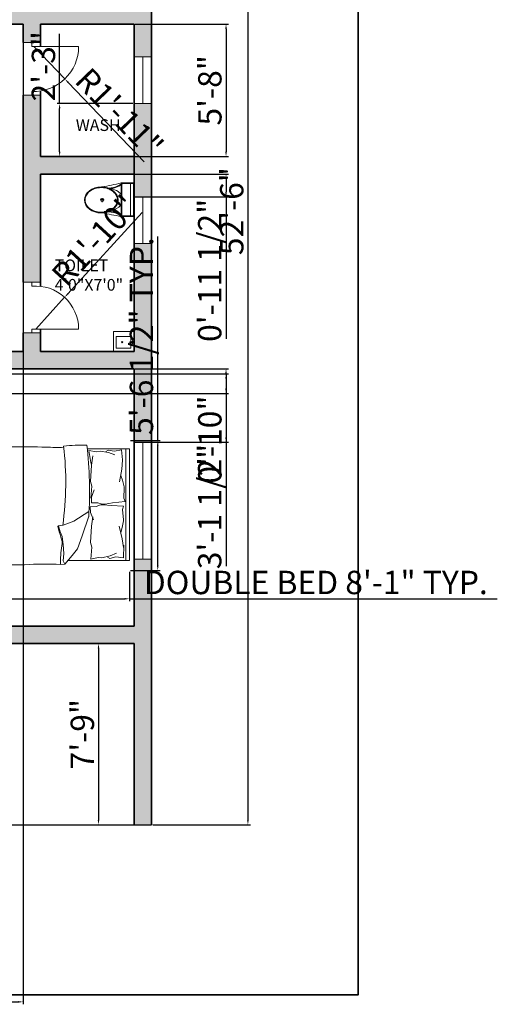
# Model space of a CAD drawing. Units: inches. Extents: x 995 to 1625, y 1005 to 1825.
# Tile 4 of 5: x 1379 to 1625, y 1015 to 1521. Entities that reach past the tile are written whole.
import ezdxf

# ---------------------------------------------------------------- set-up
doc = ezdxf.new("R2010")
doc.units = ezdxf.units.IN
for name, color, linetype, lineweight in [('A-ANNO-DIMS', 2, 'Continuous', 18), ('A-ANNO-TTLB', 7, 'Continuous', 35), ('A-AREA-IDEN', 7, 'Continuous', 18), ('A-DOOR', 4, 'Continuous', 18), ('A-FLOR-FIXT', 9, 'Continuous', 18), ('A-FURN', 8, 'Continuous', 13), ('A-GLAZ', 3, 'Continuous', 18), ('A-WALL', 7, 'Continuous', 35), ('C-PROP', 7, 'Continuous', 25)]:
    doc.layers.add(name, color=color, linetype=linetype, lineweight=lineweight)
doc.layers.add('A-WALL-PATT', color=251, linetype='Continuous', lineweight=13, true_color=0x636466)
doc.styles.get("Standard").update_dxf_attribs({"font": 'arial.ttf'})
doc.dimstyles.new('ISO-25', dxfattribs={"dimtxt": 12, "dimasz": 2.5, "dimexe": 1.25, "dimexo": 0.625, "dimtad": 1, "dimdec": 0, "dimlunit": 3, "dimtxsty": 'Standard', "dimcen": 2.5, "dimadec": 0, "dimazin": 0, "dimtfac": 1, "dimtdec": 0, "dimtmove": 0, "dimatfit": 3, "dimfxl": 1, "dimarcsym": 0})

# ---------------------------------------------------------------- blocks, each defined once
blk = doc.blocks.new('*D3')
at = {"layer": 'A-ANNO-DIMS', "color": 0, "lineweight": -2, "transparency": 16777216}
for p, q in [((1419.59, 1197.93), (1419.59, 1109.93)), ((1420.21, 1200.43), (1420.84, 1200.43)), ((1420.21, 1107.43), (1420.84, 1107.43))]:
    blk.add_line(p, q, dxfattribs=at)
at = {"layer": 'A-ANNO-DIMS', "color": 0, "transparency": 16777216}
for points in [[(1419.17, 1197.93), (1420, 1197.93), (1419.59, 1200.43)], [(1419.17, 1109.93), (1420, 1109.93), (1419.59, 1107.43)]]:
    blk.add_solid(points, dxfattribs=at)
at = {"layer": 'Defpoints', "color": 0, "transparency": 16777216}
for p in [(1419.59, 1200.43), (1419.59, 1107.43), (1419.59, 1107.43)]:
    blk.add_point(p, dxfattribs=at)
at = {"layer": 'A-ANNO-DIMS', "color": 0, "transparency": 16777216, "insert": (1412.84, 1153.93), "char_height": 12, "attachment_point": 5, "rotation": 90}
blk.add_mtext('7\'-9"', dxfattribs=at)
blk = doc.blocks.new('*D4')
at = {"layer": 'A-ANNO-DIMS', "color": 0, "lineweight": -2, "transparency": 16777216}
for p, q in [((1447.49, 1737.43), (1497.61, 1737.43)), ((1496.36, 1734.93), (1496.36, 1109.93)), ((1447.49, 1107.43), (1497.61, 1107.43))]:
    blk.add_line(p, q, dxfattribs=at)
at = {"layer": 'A-ANNO-DIMS', "color": 0, "transparency": 16777216}
for points in [[(1495.94, 1734.93), (1496.78, 1734.93), (1496.36, 1737.43)], [(1495.94, 1109.93), (1496.78, 1109.93), (1496.36, 1107.43)]]:
    blk.add_solid(points, dxfattribs=at)
at = {"layer": 'Defpoints', "color": 0, "transparency": 16777216}
for p in [(1446.87, 1737.43), (1446.87, 1107.43), (1496.36, 1107.43)]:
    blk.add_point(p, dxfattribs=at)
at = {"layer": 'A-ANNO-DIMS', "color": 0, "transparency": 16777216, "insert": (1489.61, 1422.43), "char_height": 12, "attachment_point": 5, "rotation": 90}
blk.add_mtext('52\'-6"', dxfattribs=at)
blk = doc.blocks.new('A$C31115884')
for p, q in [((283, 498), (223, 498)), ((258, 466), (258, 523)), ((0, 200), (0, 0)), ((520, 200), (0, 200)), ((10, 190), (10, 10)), ((510, 190), (10, 190)), ((510, 10), (510, 190)), ((520, 0), (520, 200)), ((510, 54), (0, 54)), ((10, 10), (510, 10)), ((0, 0), (520, 0))]:
    blk.add_line(p, q)
blk.add_circle((256, 496), 23.6)
for centre, radius, start, end in [((2778, -205), 2807, 165.4549, 171.7133), ((-295, 403), 365, 324.2091, 9.3499), ((-295, 403), 375, 324.2091, 9.3499), ((806, 403), 365, 170.6501, 215.7909), ((3237, 905), 2807, 188.2867, 194.5451), ((384, 406), 293, 190.2774, 224.1564), ((139, 406), 293, 315.8436, 2.6563), ((806, 403), 375, 179.2036, 215.7909)]:
    blk.add_arc(centre, radius, start, end)
blk.add_ellipse((256, 510), major_axis=(0, -261), ratio=0.772727)
blk.add_open_spline([(256, 259), (263, 259), (270, 260), (288, 262), (299, 265), (320, 273), (330, 278), (350, 291), (360, 299), (378, 316), (386, 326), (402, 347), (409, 358), (421, 383), (427, 395), (436, 422), (440, 436), (445, 465), (447, 480), (448, 509), (448, 524), (445, 553), (443, 568), (436, 596), (432, 610), (422, 636), (416, 649), (402, 672), (395, 683), (379, 703), (370, 712), (351, 728), (341, 735), (321, 746), (310, 751), (289, 757), (278, 759), (256, 761), (245, 761), (223, 757), (212, 754), (191, 746), (181, 741), (161, 728), (151, 720), (133, 703), (125, 693), (110, 672), (103, 660), (90, 636), (85, 623), (76, 596), (72, 582), (67, 553), (66, 538), (64, 509), (65, 494), (68, 465), (70, 450), (77, 422), (81, 408), (91, 382), (97, 370), (111, 346), (118, 335), (135, 316), (144, 307), (162, 291), (172, 284), (193, 273), (203, 269), (225, 262), (236, 260), (250, 259), (253, 259), (256, 259)], degree=3, knots=[0, 0, 0, 0, 0.110105, 0.110105, 0.285049, 0.285049, 0.459994, 0.459994, 0.634938, 0.634938, 0.809882, 0.809882, 0.984827, 0.984827, 1.159771, 1.159771, 1.334715, 1.334715, 1.50966, 1.50966, 1.684604, 1.684604, 1.859549, 1.859549, 2.034493, 2.034493, 2.209437, 2.209437, 2.384382, 2.384382, 2.559326, 2.559326, 2.73427, 2.73427, 2.909215, 2.909215, 3.084159, 3.084159, 3.259103, 3.259103, 3.434048, 3.434048, 3.608992, 3.608992, 3.783936, 3.783936, 3.958881, 3.958881, 4.133825, 4.133825, 4.30877, 4.30877, 4.483714, 4.483714, 4.658658, 4.658658, 4.833603, 4.833603, 5.008547, 5.008547, 5.183491, 5.183491, 5.358436, 5.358436, 5.53338, 5.53338, 5.708324, 5.708324, 5.883269, 5.883269, 6.058213, 6.058213, 6.233158, 6.233158, 6.283185, 6.283185, 6.283185, 6.283185])
blk = doc.blocks.new('WIN-24IN')
for p, q in [((0, 0), (0, -9)), ((24, -4.5), (24, 0)), ((24, 0), (24, -9)), ((0, -9), (0, -4.5)), ((0, -4.5), (24, -4.5))]:
    blk.add_line(p, q)
blk = doc.blocks.new('WIN-60IN')
for p, q in [((0, 0), (9, 0)), ((9, 0), (4.5, 0)), ((4.5, 0), (4.5, -60)), ((4.5, -60), (0, -60)), ((0, -60), (9, -60))]:
    blk.add_line(p, q)
blk = doc.blocks.new('BED-DOUBLE')
for p, q in [((13.64, 59.31), (35.36, 59.31)), ((15.43, 52.35), (14.57, 58.46)), ((14.57, 58.46), (18.38, 57.77)), ((16.62, 55.83), (15.82, 50.99)), ((18.38, 57.77), (20.29, 58.11)), ((20.29, 58.11), (24.62, 57.42)), ((24.45, 58.63), (23.23, 57.94)), ((27.57, 58.11), (24.45, 58.63)), ((24.62, 57.42), (27.91, 56.21)), ((31.38, 58.81), (27.57, 58.11)), ((31.35, 58.8), (31.75, 53.67)), ((33.52, 59.31), (33.52, 2.02)), ((35.36, 59.31), (35.36, 2.02)), ((15.82, 50.99), (15.3, 42.59)), ((15.82, 50.99), (15.43, 52.35)), ((31.73, 53.54), (31.38, 48.96)), ((31.75, 53.67), (31.73, 53.54)), ((31.38, 48.96), (30.17, 42.37)), ((30.86, 45.67), (31.73, 43.24)), ((-59.65, 45.42), (-59.65, 15.91)), ((15.3, 42.59), (15.97, 40.24)), ((31.73, 43.24), (32.59, 39.77)), ((15.97, 40.24), (15.49, 34.09)), ((15.86, 34.58), (17.17, 38.35)), ((32.59, 39.39), (32.42, 34.06)), ((32.59, 39.77), (32.59, 39.39)), ((15.86, 31.63), (15.86, 34.58)), ((19.07, 31.63), (15.86, 31.63)), ((20.52, 30.58), (18.31, 29.75)), ((21.33, 30.94), (19.07, 31.63)), ((22.07, 30.68), (20.52, 30.58)), ((22.89, 30.94), (21.33, 30.94)), ((25.92, 30.23), (22.07, 30.68)), ((26.7, 31.63), (22.89, 30.94)), ((33.11, 32.33), (26.7, 31.63)), ((32.42, 34.06), (33.11, 32.33)), ((14.51, 27.2), (6.73, 22.18)), ((18.31, 29.75), (15.1, 29.55)), ((15.1, 29.55), (15.29, 26.61)), ((15.29, 26.61), (16.83, 22.93)), ((32.37, 29.94), (25.92, 30.23)), ((31.78, 28.16), (32.37, 29.94)), ((32.29, 22.85), (31.78, 28.16)), ((6.73, 22.18), (1.35, 20.13)), ((11, 14.75), (14.51, 24.75)), ((16.62, 24.44), (15.82, 19.6)), ((31.66, 18.96), (32.31, 22.47)), ((32.31, 22.47), (32.29, 22.85)), ((1.35, 20.13), (-1.06, 19.76)), ((-1.06, 19.76), (-0.32, 16.79)), ((-0.32, 16.79), (0.79, 14.38)), ((15.82, 19.6), (15.3, 11.2)), ((31.68, 13.23), (30.05, 19.72)), ((30.95, 16.48), (31.66, 18.96)), ((0.79, 14.38), (1.35, 10.29)), ((1.35, 10.29), (1.72, 5.65)), ((8.59, 8.07), (11, 14.75)), ((15.3, 11.2), (15.97, 8.85)), ((32.31, 8.67), (31.68, 13.23)), ((1.72, 5.65), (1.35, 1.94)), ((5.99, 4.54), (8.59, 8.07)), ((15.97, 8.85), (15.49, 2.7)), ((25.46, 4.36), (28.67, 5.78)), ((32.29, 3.4), (32.41, 9.88)), ((32.41, 9.88), (32.31, 8.67)), ((0, 0), (2.09, 0.1, 4.64)), ((1.35, 1.94), (2.09, 0.1)), ((2.09, 0.1), (5.99, 4.54)), ((35.36, 2.02), (3.45, 2.02)), ((15.49, 2.7), (19.25, 3.63)), ((19.25, 3.63), (21.17, 3.4)), ((21.17, 3.4), (25.46, 4.36)), ((25.36, 3.14), (24.1, 3.76)), ((28.44, 3.85), (25.36, 3.14)), ((32.29, 3.4), (28.44, 3.85))]:
    blk.add_line(p, q)
for centre, radius, start, end in [((-60.22, 62.17), 1.31, 56.1736, 203.4781), ((-205.42, 37.79), 145.97, 2.9958, 9.4091), ((-48.9, 89.44), 28.25, 247.9751, 266.652), ((-41.99, 95.72), 35.53, 256.0648, 268.9113), ((-152.05, 42.19), 154.68, 351.7845, 6.9006), ((11.26, -38.62), 99.87, 88.7218, 95.604), ((-182.9, 37.87), 197.77, 356.0865, 6.7821), ((-25.32, -517.76), 578.22, 88.22771, 91.71854), ((-2.02, 264.05), 203.94, 268.4762, 271.0082), ((63.78, 84.12), 127.63, 193.3832, 197.7053), ((-219.13, 14.14), 159.5, 354.4998, 0.6351), ((-1.14, 19.55), 0.221, 70.2464, 181.1377), ((33.58, 26.13), 35.55, 190.6617, 199.8806), ((-6.68, 11.03), 7.46, 348.6608, 23.7384), ((43.33, 1.94), 43.38, 169.8763, 182.5657), ((-8.18, -155.03), 155.25, 86.9791, 93.8365), ((-46.97, -27.83), 27.65, 87.4714, 116.4681), ((-45.95, 5468.82), 5469.02, 270.00217, 270.28689)]:
    blk.add_arc(centre, radius, start, end)
blk = doc.blocks.new('*D18')
at = {"layer": 'A-ANNO-DIMS', "color": 0, "lineweight": -2, "transparency": 16777216}
for p, q in [((1338.5, 1237.34), (1338.5, 1222.16)), ((1435.5, 1237.34), (1435.5, 1222.16)), ((1341, 1223.41), (1433, 1223.41)), ((1435.5, 1223.41), (1624.52, 1223.41))]:
    blk.add_line(p, q, dxfattribs=at)
at = {"layer": 'A-ANNO-DIMS', "color": 0, "transparency": 16777216}
for points in [[(1341, 1223.83), (1341, 1223), (1338.5, 1223.41)], [(1433, 1223.83), (1433, 1223), (1435.5, 1223.41)]]:
    blk.add_solid(points, dxfattribs=at)
at = {"layer": 'Defpoints', "color": 0, "transparency": 16777216}
for p in [(1338.5, 1237.96), (1435.5, 1237.96), (1435.5, 1223.41)]:
    blk.add_point(p, dxfattribs=at)
at = {"layer": 'A-ANNO-DIMS', "color": 0, "transparency": 16777216, "insert": (1531.26, 1230.25), "char_height": 12, "attachment_point": 5}
blk.add_mtext('DOUBLE BED 8\'-1" TYP.', dxfattribs=at)
blk = doc.blocks.new('*D19')
at = {"layer": 'A-ANNO-DIMS', "color": 0, "lineweight": -2, "transparency": 16777216}
for p, q in [((1450.05, 1304.62), (1450.05, 1409.47)), ((1436.12, 1304.62), (1451.3, 1304.62)), ((1450.05, 1240.46), (1450.05, 1302.12)), ((1436.12, 1237.96), (1451.3, 1237.96))]:
    blk.add_line(p, q, dxfattribs=at)
at = {"layer": 'A-ANNO-DIMS', "color": 0, "transparency": 16777216}
for points in [[(1449.63, 1302.12), (1450.46, 1302.12), (1450.05, 1304.62)], [(1449.63, 1240.46), (1450.46, 1240.46), (1450.05, 1237.96)]]:
    blk.add_solid(points, dxfattribs=at)
at = {"layer": 'Defpoints', "color": 0, "transparency": 16777216}
for p in [(1435.5, 1304.62), (1450.05, 1304.62), (1435.5, 1237.96)]:
    blk.add_point(p, dxfattribs=at)
at = {"layer": 'A-ANNO-DIMS', "color": 0, "transparency": 16777216, "insert": (1443.22, 1358.29), "char_height": 12, "attachment_point": 5, "rotation": 90}
blk.add_mtext('5\'-6 1/2" TYP.', dxfattribs=at)
blk = doc.blocks.new('*D26')
at = {"layer": 'A-ANNO-DIMS', "color": 0, "lineweight": -2, "transparency": 16777216}
for p, q in [((1076.49, 1338.88), (1486.37, 1338.88)), ((1485.12, 1336.38), (1485.12, 1331.38)), ((1076.49, 1328.88), (1486.37, 1328.88)), ((1485.12, 1328.88), (1485.12, 1283.91))]:
    blk.add_line(p, q, dxfattribs=at)
at = {"layer": 'A-ANNO-DIMS', "color": 0, "transparency": 16777216}
for points in [[(1484.7, 1336.38), (1485.53, 1336.38), (1485.12, 1338.88)], [(1484.7, 1331.38), (1485.53, 1331.38), (1485.12, 1328.88)]]:
    blk.add_solid(points, dxfattribs=at)
at = {"layer": 'Defpoints', "color": 0, "transparency": 16777216}
for p in [(1075.87, 1338.88), (1075.87, 1328.88), (1485.12, 1328.88)]:
    blk.add_point(p, dxfattribs=at)
at = {"layer": 'A-ANNO-DIMS', "color": 0, "transparency": 16777216, "insert": (1478.36, 1305.15), "char_height": 12, "attachment_point": 5, "rotation": 90}
blk.add_mtext('0\'-10"', dxfattribs=at)
blk = doc.blocks.new('*D28')
at = {"layer": 'A-ANNO-DIMS', "color": 0, "lineweight": -2, "transparency": 16777216}
for p, q in [((1438.49, 1518.43), (1486.37, 1518.43)), ((1485.12, 1515.93), (1485.12, 1452.93)), ((1438.49, 1450.43), (1486.37, 1450.43))]:
    blk.add_line(p, q, dxfattribs=at)
at = {"layer": 'A-ANNO-DIMS', "color": 0, "transparency": 16777216}
for points in [[(1484.7, 1515.93), (1485.53, 1515.93), (1485.12, 1518.43)], [(1484.7, 1452.93), (1485.53, 1452.93), (1485.12, 1450.43)]]:
    blk.add_solid(points, dxfattribs=at)
at = {"layer": 'Defpoints', "color": 0, "transparency": 16777216}
for p in [(1437.87, 1518.43), (1437.87, 1450.43), (1485.12, 1450.43)]:
    blk.add_point(p, dxfattribs=at)
at = {"layer": 'A-ANNO-DIMS', "color": 0, "transparency": 16777216, "insert": (1478.36, 1484.43), "char_height": 12, "attachment_point": 5, "rotation": 90}
blk.add_mtext('5\'-8"', dxfattribs=at)
blk = doc.blocks.new('*D29')
at = {"layer": 'A-ANNO-DIMS', "color": 0, "lineweight": -2, "transparency": 16777216}
for p, q in [((1380.24, 1518.43), (1341.37, 1518.43)), ((1342.62, 1352.93), (1342.62, 1515.93)), ((1380.24, 1350.43), (1341.37, 1350.43))]:
    blk.add_line(p, q, dxfattribs=at)
at = {"layer": 'A-ANNO-DIMS', "color": 0, "transparency": 16777216}
for points in [[(1342.2, 1515.93), (1343.03, 1515.93), (1342.62, 1518.43)], [(1342.2, 1352.93), (1343.03, 1352.93), (1342.62, 1350.43)]]:
    blk.add_solid(points, dxfattribs=at)
at = {"layer": 'Defpoints', "color": 0, "transparency": 16777216}
for p in [(1342.62, 1518.43), (1380.87, 1518.43), (1380.87, 1350.43)]:
    blk.add_point(p, dxfattribs=at)
at = {"layer": 'A-ANNO-DIMS', "color": 0, "transparency": 16777216, "insert": (1335.86, 1434.43), "char_height": 12, "attachment_point": 5, "rotation": 90}
blk.add_mtext('14\'-0"', dxfattribs=at)
blk = doc.blocks.new('*D30')
at = {"layer": 'A-ANNO-DIMS', "color": 0, "lineweight": -2, "transparency": 16777216}
for p, q in [((1212.87, 1517.8), (1212.87, 1015.27)), ((1380.87, 1517.8), (1380.87, 1015.27)), ((1215.37, 1016.52), (1378.37, 1016.52))]:
    blk.add_line(p, q, dxfattribs=at)
at = {"layer": 'A-ANNO-DIMS', "color": 0, "transparency": 16777216}
for points in [[(1215.37, 1016.93), (1215.37, 1016.1), (1212.87, 1016.52)], [(1378.37, 1016.93), (1378.37, 1016.1), (1380.87, 1016.52)]]:
    blk.add_solid(points, dxfattribs=at)
at = {"layer": 'Defpoints', "color": 0, "transparency": 16777216}
for p in [(1212.87, 1518.43), (1380.87, 1518.43), (1380.87, 1016.52)]:
    blk.add_point(p, dxfattribs=at)
at = {"layer": 'A-ANNO-DIMS', "color": 0, "transparency": 16777216, "insert": (1296.87, 1023.27), "char_height": 12, "attachment_point": 5}
blk.add_mtext('14\'-0"', dxfattribs=at)
blk = doc.blocks.new('*D39')
at = {"layer": 'A-ANNO-DIMS', "color": 0, "lineweight": -2, "transparency": 16777216}
for p, q in [((1399.62, 1477.62), (1399.62, 1513.47)), ((1437.24, 1477.62), (1398.37, 1477.62)), ((1399.62, 1452.93), (1399.62, 1475.12)), ((1437.24, 1450.43), (1398.37, 1450.43))]:
    blk.add_line(p, q, dxfattribs=at)
at = {"layer": 'A-ANNO-DIMS', "color": 0, "transparency": 16777216}
for points in [[(1399.2, 1475.12), (1400.03, 1475.12), (1399.62, 1477.62)], [(1399.2, 1452.93), (1400.03, 1452.93), (1399.62, 1450.43)]]:
    blk.add_solid(points, dxfattribs=at)
at = {"layer": 'Defpoints', "color": 0, "transparency": 16777216}
for p in [(1399.62, 1477.62), (1437.87, 1477.62), (1437.87, 1450.43)]:
    blk.add_point(p, dxfattribs=at)
at = {"layer": 'A-ANNO-DIMS', "color": 0, "transparency": 16777216, "insert": (1392.86, 1496.79), "char_height": 12, "attachment_point": 5, "rotation": 90}
blk.add_mtext('2\'-3"', dxfattribs=at)
blk = doc.blocks.new('*D40')
at = {"layer": 'A-ANNO-DIMS', "color": 0, "lineweight": -2, "transparency": 16777216}
for p, q in [((1438.49, 1441.43), (1486.37, 1441.43)), ((1485.12, 1438.93), (1485.12, 1432.25)), ((1438.49, 1429.75), (1486.37, 1429.75)), ((1485.12, 1429.75), (1485.12, 1356.81))]:
    blk.add_line(p, q, dxfattribs=at)
at = {"layer": 'A-ANNO-DIMS', "color": 0, "transparency": 16777216}
for points in [[(1484.7, 1438.93), (1485.53, 1438.93), (1485.12, 1441.43)], [(1484.7, 1432.25), (1485.53, 1432.25), (1485.12, 1429.75)]]:
    blk.add_solid(points, dxfattribs=at)
at = {"layer": 'Defpoints', "color": 0, "transparency": 16777216}
for p in [(1437.87, 1441.43), (1437.87, 1429.75), (1485.12, 1429.75)]:
    blk.add_point(p, dxfattribs=at)
at = {"layer": 'A-ANNO-DIMS', "color": 0, "transparency": 16777216, "insert": (1478.29, 1392.03), "char_height": 12, "attachment_point": 5, "rotation": 90}
blk.add_mtext('0\'-11 1/2"', dxfattribs=at)
blk = doc.blocks.new('*D41')
at = {"layer": 'A-ANNO-DIMS', "color": 0, "lineweight": -2, "transparency": 16777216}
for p, q in [((1438.49, 1341.43), (1486.37, 1341.43)), ((1485.12, 1338.93), (1485.12, 1306.34)), ((1438.49, 1303.84), (1486.37, 1303.84)), ((1485.12, 1303.84), (1485.12, 1240.24))]:
    blk.add_line(p, q, dxfattribs=at)
at = {"layer": 'A-ANNO-DIMS', "color": 0, "transparency": 16777216}
for points in [[(1484.7, 1338.93), (1485.53, 1338.93), (1485.12, 1341.43)], [(1484.7, 1306.34), (1485.53, 1306.34), (1485.12, 1303.84)]]:
    blk.add_solid(points, dxfattribs=at)
at = {"layer": 'Defpoints', "color": 0, "transparency": 16777216}
for p in [(1437.87, 1341.43), (1437.87, 1303.84), (1485.12, 1303.84)]:
    blk.add_point(p, dxfattribs=at)
at = {"layer": 'A-ANNO-DIMS', "color": 0, "transparency": 16777216, "insert": (1478.28, 1270.79), "char_height": 12, "attachment_point": 5, "rotation": 90}
blk.add_mtext('3\'-1 1/2"', dxfattribs=at)
blk = doc.blocks.new('*D51')
at = {"layer": 'A-ANNO-DIMS', "color": 0, "lineweight": -2, "transparency": 16777216}
for p, q in [((1386.31, 1506.92), (1402.28, 1490.28)), ((1443.11, 1447.75), (1404.01, 1488.48))]:
    blk.add_line(p, q, dxfattribs=at)
at = {"layer": 'A-ANNO-DIMS', "color": 0, "transparency": 16777216}
blk.add_solid([(1404.31, 1488.77), (1403.71, 1488.19), (1402.28, 1490.28)], dxfattribs=at)
at = {"layer": 'Defpoints', "color": 0, "transparency": 16777216}
for p in [(1386.31, 1506.92), (1402.28, 1490.28)]:
    blk.add_point(p, dxfattribs=at)
at = {"layer": 'A-ANNO-DIMS', "color": 0, "transparency": 16777216, "insert": (1429.22, 1471.82), "char_height": 12, "attachment_point": 5, "rotation": 313.833}
blk.add_mtext('R1\'-11"', dxfattribs=at)
blk = doc.blocks.new('*D53')
at = {"layer": 'A-ANNO-DIMS', "color": 0, "lineweight": -2, "transparency": 16777216}
for p, q in [((1442.01, 1421.66), (1403.89, 1380.02)), ((1387.31, 1361.9), (1402.2, 1378.17))]:
    blk.add_line(p, q, dxfattribs=at)
at = {"layer": 'A-ANNO-DIMS', "color": 0, "transparency": 16777216}
blk.add_solid([(1403.58, 1380.3), (1404.2, 1379.74), (1402.2, 1378.17)], dxfattribs=at)
at = {"layer": 'Defpoints', "color": 0, "transparency": 16777216}
for p in [(1402.2, 1378.17), (1387.31, 1361.9)]:
    blk.add_point(p, dxfattribs=at)
at = {"layer": 'A-ANNO-DIMS', "color": 0, "transparency": 16777216, "insert": (1418.82, 1406.32), "char_height": 12, "attachment_point": 5, "rotation": 47.5256}
blk.add_mtext('R1\'-10"', dxfattribs=at)

msp = doc.modelspace()

# ---------------------------------------------------------------- hatches: boundary and pattern name
at = {"layer": 'A-WALL-PATT'}
h = msp.add_hatch(color=256, dxfattribs=at)
h.dxf.hatch_style = 1
h.paths.add_polyline_path([(1446.87, 1737.43), (1066.87, 1737.43), (1066.87, 1718.28), (1075.87, 1718.28), (1075.87, 1728.43), (1171.87, 1728.43), (1171.87, 1668.43), (1165.05, 1668.43), (1165.05, 1659.43), (1219.13, 1659.43), (1219.13, 1663.93), (1219.13, 1668.43), (1180.87, 1668.43), (1180.87, 1691.88), (1180.87, 1728.43), (1249.87, 1728.43), (1258.87, 1728.43), (1332.87, 1728.43), (1332.87, 1668.43), (1311.16, 1668.43), (1311.16, 1659.43), (1346.35, 1659.43), (1346.35, 1663.93), (1346.35, 1668.43), (1341.87, 1668.43), (1341.87, 1728.43), (1437.87, 1728.43), (1437.87, 1715.56), (1446.87, 1715.56)])
h.paths.add_polyline_path([(1135.58, 1663.93), (1135.58, 1668.43), (1075.87, 1668.43), (1075.87, 1694.28), (1066.87, 1694.28), (1066.87, 1619.54), (1075.87, 1619.54), (1075.87, 1659.43), (1135.58, 1659.43)])
h.paths.add_polyline_path([(1258.87, 1659.43), (1275.16, 1659.43), (1275.16, 1663.93), (1275.16, 1668.43), (1258.87, 1668.43), (1249.87, 1668.43), (1243.74, 1668.43), (1243.74, 1659.43), (1249.87, 1659.43), (1249.87, 1527.43), (1247.75, 1527.43), (1247.75, 1518.43), (1261.81, 1518.43), (1261.81, 1527.43), (1258.87, 1527.43)])
h.paths.add_polyline_path([(1446.87, 1691.56), (1437.87, 1691.56), (1437.87, 1668.43), (1372.6, 1668.43), (1372.6, 1659.43), (1437.87, 1659.43), (1437.87, 1627.58), (1446.87, 1627.58)])
h.paths.add_polyline_path([(1446.87, 1567.58), (1437.87, 1567.58), (1437.87, 1527.43), (1291.03, 1527.43), (1291.03, 1518.43), (1380.87, 1518.43), (1380.87, 1508.92), (1389.87, 1508.92), (1389.87, 1518.43), (1437.87, 1518.43), (1437.87, 1501.62), (1446.87, 1501.62)])
h.paths.add_polyline_path([(1446.87, 1477.62), (1437.87, 1477.62), (1437.87, 1429.75), (1446.87, 1429.75)])
h.paths.add_polyline_path([(1389.87, 1441.43), (1437.87, 1441.43), (1437.87, 1450.43), (1389.87, 1450.43), (1389.87, 1481.88), (1385.37, 1481.88), (1380.87, 1481.88), (1380.87, 1385.88), (1389.87, 1385.88)])
h.paths.add_polyline_path([(1446.87, 1405.75), (1437.87, 1405.75), (1437.87, 1350.43), (1427.33, 1350.43), (1389.87, 1350.43), (1389.87, 1359.9), (1380.87, 1359.9), (1380.87, 1350.43), (1324.85, 1350.43), (1324.85, 1341.43), (1437.87, 1341.43), (1437.87, 1303.84), (1446.87, 1303.84)])
h.paths.add_polyline_path([(1311.82, 1209.43), (1281.87, 1209.43), (1281.87, 1341.43), (1291.29, 1341.43), (1291.29, 1345.93), (1291.29, 1350.43), (1244.83, 1350.43), (1244.83, 1341.43), (1272.87, 1341.43), (1272.87, 1185.43), (1268.73, 1185.43), (1268.73, 1176.43), (1272.87, 1176.43), (1281.87, 1176.43), (1281.87, 1200.43), (1311.82, 1200.43), (1311.82, 1204.93)])
h.paths.add_polyline_path([(1446.87, 1243.84), (1437.87, 1243.84), (1437.87, 1209.43), (1371.82, 1209.43), (1371.82, 1200.43), (1437.87, 1200.43), (1437.87, 1107.43), (1446.87, 1107.43)])
h.paths.add_polyline_path([(1212.11, 1185.43), (1207.85, 1185.43), (1207.85, 1176.43), (1212.11, 1176.43)], flags=17)
h.paths.add_polyline_path([(1244.73, 1185.43), (1240.24, 1185.43), (1240.24, 1176.43), (1244.73, 1176.43), (1244.73, 1180.93)])
h.paths.add_polyline_path([(1183.85, 1180.93), (1183.85, 1185.43), (1180.87, 1185.43), (1180.87, 1191.84), (1171.87, 1191.84), (1171.87, 1176.43), (1180.87, 1176.43), (1183.85, 1176.43)], flags=17)
h.paths.add_polyline_path([(1180.87, 1341.43), (1198.57, 1341.43), (1198.57, 1350.43), (1180.87, 1350.43), (1180.87, 1354.13), (1176.37, 1354.13), (1171.87, 1354.13), (1171.87, 1341.43), (1171.87, 1219.68), (1180.87, 1219.68)], flags=17)
h.paths.add_polyline_path([(1075.87, 1391.93), (1171.87, 1391.93), (1171.87, 1389.24), (1180.87, 1389.24), (1180.87, 1391.93), (1212.87, 1391.93), (1212.87, 1431.83), (1203.87, 1431.83), (1203.87, 1400.93), (1075.87, 1400.93), (1075.87, 1446.29), (1066.87, 1446.29), (1066.87, 1107.43), (1075.87, 1107.43)])
h.paths.add_polyline_path([(1218.33, 1527.43), (1075.87, 1527.43), (1075.87, 1559.54), (1066.87, 1559.54), (1066.87, 1482.29), (1075.87, 1482.29), (1075.87, 1518.43), (1203.87, 1518.43), (1203.87, 1493.65), (1212.87, 1493.65), (1212.87, 1518.43), (1218.33, 1518.43), (1218.33, 1522.93)])
h.paths.add_polyline_path([(1297.68, 1457.37), (1297.68, 1425.03), (1310.04, 1425.03), (1310.04, 1457.37)], flags=9)
h.paths.add_polyline_path([(1154.86, 1054.62), (1346.22, 1054.62), (1346.22, 1079.35), (1154.86, 1079.35)], flags=9)
h.paths.add_polyline_path([(1237.85, 1265.85), (1262.06, 1265.85), (1262.06, 1288.24), (1237.85, 1288.24)], flags=9)
h.paths.add_polyline_path([(1331.39, 1305.41), (1378, 1305.41), (1378, 1327.8), (1331.39, 1327.8)], flags=25)
h.paths.add_polyline_path([(1395.38, 1378.18), (1431.86, 1378.18), (1431.86, 1400.57), (1395.38, 1400.57)], flags=25)
h.paths.add_polyline_path([(1406.34, 1460.18), (1434.48, 1460.18), (1434.48, 1472.55), (1406.34, 1472.55)], flags=25)
h.paths.add_polyline_path([(1134.66, 1454.9), (1180.38, 1454.9), (1180.38, 1477.29), (1134.66, 1477.29)], flags=9)
h.paths.add_polyline_path([(1109.63, 1626.32), (1156.23, 1626.32), (1156.23, 1648.71), (1109.63, 1648.71)], flags=9)
h.paths.add_polyline_path([(1275.64, 1623.22), (1322.25, 1623.22), (1322.25, 1645.61), (1275.64, 1645.61)], flags=9)
h.paths.add_polyline_path([(1347.7, 1693.6), (1384.09, 1693.6), (1384.09, 1715.99), (1347.7, 1715.99)], flags=25)
h.paths.add_polyline_path([(1254.21, 1701.46), (1308.94, 1701.46), (1308.94, 1723.85), (1254.21, 1723.85)], flags=25)
h.paths.add_polyline_path([(1107.35, 1692.25), (1143.74, 1692.25), (1143.74, 1714.64), (1107.35, 1714.64)], flags=25)

# ---------------------------------------------------------------- linework, layer by layer
at = {"layer": 'A-ANNO-TTLB'}
msp.add_lwpolyline([(995.18, 1825.14), (1553.05, 1825.14), (1553.05, 1020.2), (995.18, 1020.2)], close=True, dxfattribs=at)
at = {"layer": 'A-DOOR'}
for p, q in [((1380.87, 1508.92), (1389.87, 1508.92)), ((1389.87, 1508.92), (1385.37, 1508.92)), ((1385.37, 1508.92), (1385.37, 1506.92)), ((1385.37, 1506.92), (1409.37, 1506.92)), ((1380.87, 1481.88), (1389.87, 1481.88)), ((1385.37, 1481.88), (1385.37, 1483.88)), ((1389.87, 1481.88), (1385.37, 1481.88)), ((1380.87, 1385.88), (1389.87, 1385.88)), ((1389.87, 1385.88), (1385.37, 1385.88)), ((1385.37, 1385.88), (1385.37, 1383.88)), ((1380.87, 1359.9), (1389.87, 1359.9)), ((1385.37, 1359.9), (1385.37, 1361.9)), ((1385.37, 1361.9), (1409.37, 1361.9)), ((1389.87, 1359.9), (1389.87, 1359.9))]:
    msp.add_line(p, q, dxfattribs=at)
for centre, radius, start, end in [((1386.31, 1506.92), 23.06, 267.6655, 360), ((1387.31, 1361.9), 22.06, 360, 95.0495)]:
    msp.add_arc(centre, radius, start, end, dxfattribs=at)
at = {"layer": 'A-FLOR-FIXT'}
msp.add_lwpolyline([(1427.33, 1360.55), (1437.87, 1360.55), (1437.87, 1350.43), (1427.33, 1350.43)], close=True, dxfattribs=at)
for points in [[(1436.24, 1354.76), (1436.24, 1352.06), (1428.69, 1352.06), (1428.69, 1357.98), (1436.24, 1357.98), (1436.24, 1355.28)], [(1436.84, 1354.76), (1435.65, 1354.76), (1435.65, 1355.28), (1436.84, 1355.28)], [(1436.84, 1355.28), (1436.84, 1355.59), (1437.16, 1355.59), (1437.16, 1354.51), (1436.84, 1354.51), (1436.84, 1354.76)]]:
    msp.add_lwpolyline(points, dxfattribs=at)
msp.add_circle((1431.76, 1355.18), 0.287, dxfattribs=at)
at = {"layer": 'A-WALL'}
for p, q in [((1446.87, 1737.43), (1446.87, 1107.43)), ((1291.03, 1518.43), (1380.87, 1518.43)), ((1380.87, 1518.43), (1380.87, 1508.92)), ((1389.87, 1518.43), (1389.87, 1506.92)), ((1389.87, 1518.43), (1437.87, 1518.43)), ((1437.87, 1518.43), (1437.87, 1350.43)), ((1380.87, 1481.88), (1380.87, 1385.88)), ((1389.87, 1484.13), (1389.87, 1450.43)), ((1380.87, 1441.43), (1380.87, 1450.43)), ((1389.87, 1450.43), (1437.87, 1450.43)), ((1437.87, 1441.43), (1389.87, 1441.43)), ((1389.87, 1441.43), (1389.87, 1383.81)), ((1437.87, 1350.43), (1437.87, 1441.43)), ((1380.87, 1359.9), (1380.87, 1350.43)), ((1389.87, 1361.9), (1389.87, 1350.43)), ((1324.85, 1350.43), (1380.87, 1350.43)), ((1389.87, 1350.43), (1437.87, 1350.43)), ((1323.4, 1341.43), (1437.87, 1341.43)), ((1437.87, 1341.43), (1437.87, 1209.43)), ((1281.87, 1209.43), (1437.87, 1209.43)), ((1281.87, 1200.43), (1437.87, 1200.43)), ((1437.87, 1200.43), (1437.87, 1107.43))]:
    msp.add_line(p, q, dxfattribs=at)
at = {"layer": 'C-PROP'}
msp.add_line((1066.87, 1107.43), (1446.87, 1107.43), dxfattribs=at)

# ---------------------------------------------------------------- block references
at = {"layer": 'A-FLOR-FIXT', "xscale": 0.0330640103915726, "yscale": 0.0330640103915726, "zscale": 0.0330640103915726, "rotation": 89.99999999999991}
msp.add_blockref('A$C31115884', (1437.87, 1419.69), dxfattribs=at)
at = {"layer": 'A-FURN'}
msp.add_blockref('BED-DOUBLE', (1400.14, 1241.04), dxfattribs=at)
at = {"layer": 'A-GLAZ', "extrusion": (0, 0, -1), "zscale": -1}
for p, rotation in [((-1437.87, 1501.62), 269.9999999999928), ((-1437.87, 1429.75), 270)]:
    msp.add_blockref('WIN-24IN', p, dxfattribs=dict(at, rotation=rotation))
at = {"layer": 'A-GLAZ'}
msp.add_blockref('WIN-60IN', (1437.87, 1303.84), dxfattribs=at)

# ---------------------------------------------------------------- texts
at = {"layer": 'A-AREA-IDEN', "char_height": 6, "attachment_point": 1}
for s, width, insert in [('WASH', 76.0838, (1407.94, 1469.56)), ('TOILET\\P4\'0"X7\'0"', 95.7312, (1397.08, 1397.59))]:
    msp.add_mtext_dynamic_manual_height_columns(s, width=width, gutter_width=12.5, heights=[0], dxfattribs=dict(at, insert=insert))

# ---------------------------------------------------------------- dimensions: what is measured, and where the dimension line sits
at = {"layer": 'A-ANNO-DIMS'}
for base, p1, p2, override, picture, middle in [((1496.36, 1107.43), (1446.87, 1737.43), (1446.87, 1107.43), {"dimclrd": 0, "dimclre": 0, "dimclrt": 0}, '*D4', (1489.61, 1422.43)), ((1342.62, 1518.43), (1380.87, 1350.43), (1380.87, 1518.43), {"dimdec": 1, "dimlfac": 1, "dimrnd": 0, "dimzin": 1, "dimdsep": 46, "dimlunit": 4, "dimfrac": 2}, '*D29', (1335.86, 1434.43)), ((1485.12, 1450.43), (1437.87, 1518.43), (1437.87, 1450.43), {"dimdec": 1, "dimlfac": 1, "dimrnd": 0, "dimzin": 1, "dimdsep": 46, "dimlunit": 4, "dimfrac": 2}, '*D28', (1478.36, 1484.43)), ((1399.62, 1477.62), (1437.87, 1450.43), (1437.87, 1477.62), {"dimdec": 1, "dimlfac": 1, "dimrnd": 0, "dimzin": 1, "dimdsep": 46, "dimlunit": 4, "dimfrac": 2}, '*D39', (1392.86, 1496.79)), ((1485.12, 1429.75), (1437.87, 1441.43), (1437.87, 1429.75), {"dimdec": 1, "dimlfac": 1, "dimrnd": 0, "dimzin": 1, "dimdsep": 46, "dimlunit": 4, "dimfrac": 2}, '*D40', (1478.29, 1392.03)), ((1485.12, 1303.84), (1437.87, 1341.43), (1437.87, 1303.84), {"dimdec": 1, "dimlfac": 1, "dimrnd": 0, "dimzin": 1, "dimdsep": 46, "dimlunit": 4, "dimfrac": 2}, '*D41', (1478.28, 1270.79)), ((1485.12, 1328.88), (1075.87, 1338.88), (1075.87, 1328.88), {"dimdec": 1, "dimlfac": 1, "dimrnd": 0, "dimzin": 1, "dimdsep": 46, "dimlunit": 4, "dimfrac": 2}, '*D26', (1478.36, 1305.15)), ((1419.59, 1107.43), (1419.59, 1200.43), (1419.59, 1107.43), {"dimclrd": 0, "dimclre": 0, "dimclrt": 0}, '*D3', (1412.84, 1153.93))]:
    dim = msp.add_linear_dim(base=base, p1=p1, p2=p2, angle=90, dimstyle='ISO-25', override=override, dxfattribs=at)
    dim.commit()
    dim.dimension.update_dxf_attribs({"geometry": picture, "text_midpoint": middle})
dim = msp.add_linear_dim(base=(1380.87, 1016.52), p1=(1212.87, 1518.43), p2=(1380.87, 1518.43), dimstyle='ISO-25', override={"dimdec": 1, "dimlfac": 1, "dimrnd": 0, "dimzin": 1, "dimdsep": 46, "dimlunit": 4, "dimfrac": 2}, dxfattribs=at)
dim.commit()
dim.dimension.update_dxf_attribs({"geometry": '*D30', "text_midpoint": (1296.87, 1023.27)})
for center, mpoint, picture, middle in [((1386.31, 1506.92), (1402.28, 1490.28), '*D51', (1429.22, 1471.82)), ((1387.31, 1361.9), (1402.2, 1378.17), '*D53', (1418.82, 1406.32))]:
    dim = msp.add_radius_dim(center=center, mpoint=mpoint, dimstyle='ISO-25', override={"dimdec": 1, "dimlfac": 1, "dimrnd": 0, "dimzin": 1, "dimdsep": 46, "dimlunit": 4, "dimfrac": 2}, dxfattribs=at)
    dim.commit()
    dim.dimension.update_dxf_attribs({"geometry": picture, "text_midpoint": middle})
dim = msp.add_linear_dim(base=(1450.05, 1304.62), p1=(1435.5, 1237.96), p2=(1435.5, 1304.62), angle=90, text='<> TYP.', dimstyle='ISO-25', override={"dimdec": 1, "dimlfac": 1, "dimrnd": 0, "dimzin": 1, "dimdsep": 46, "dimlunit": 4, "dimfrac": 2}, dxfattribs=at)
dim.commit()
dim.dimension.update_dxf_attribs({"geometry": '*D19', "text_midpoint": (1443.22, 1358.29)})
dim = msp.add_linear_dim(base=(1435.5, 1223.41), p1=(1338.5, 1237.96), p2=(1435.5, 1237.96), text='DOUBLE BED <> TYP.', dimstyle='ISO-25', override={"dimdec": 1, "dimlfac": 1, "dimrnd": 0, "dimzin": 1, "dimdsep": 46, "dimlunit": 4, "dimfrac": 2}, dxfattribs=at)
dim.commit()
dim.dimension.update_dxf_attribs({"geometry": '*D18', "text_midpoint": (1531.26, 1230.25)})

doc.saveas('drawing.dxf')
